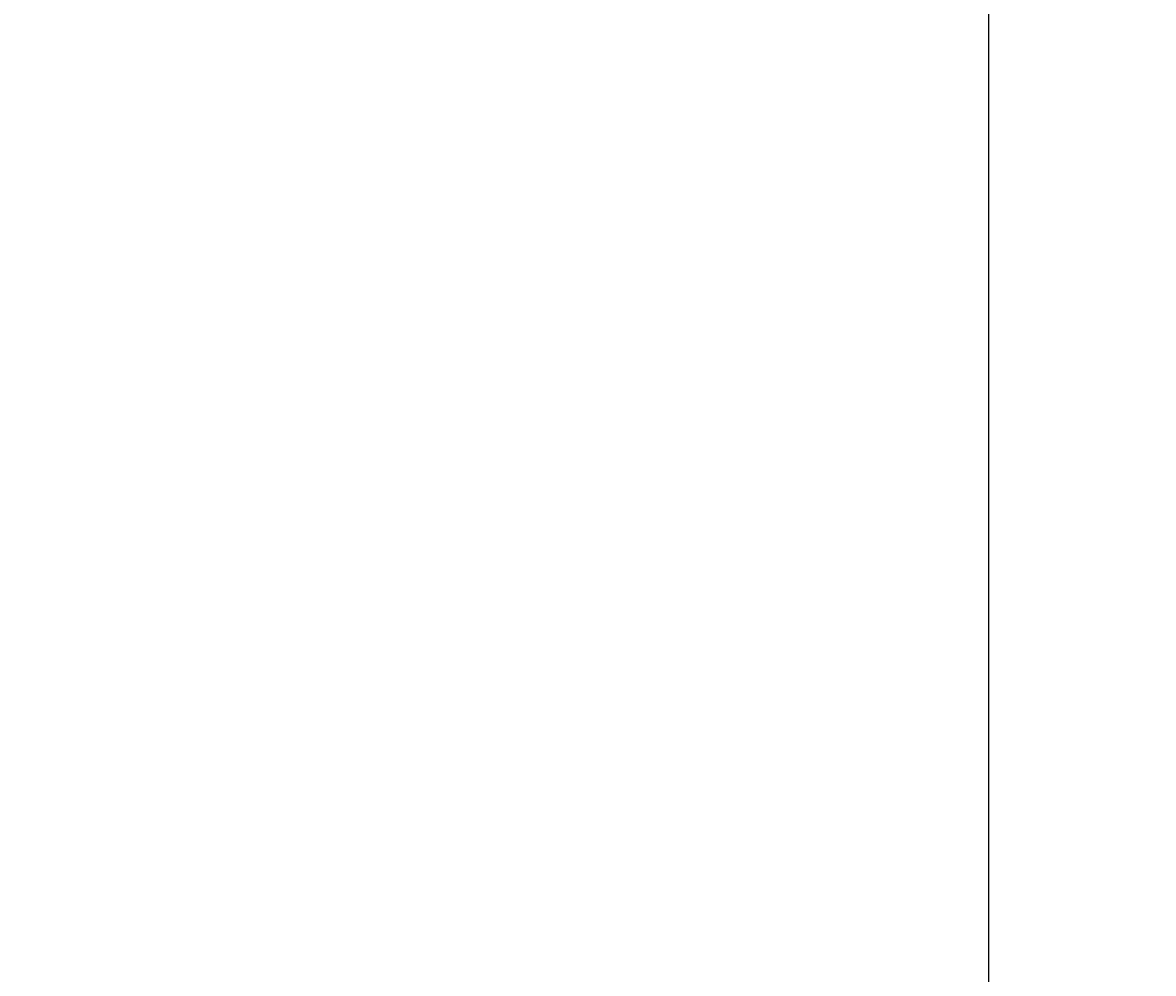
# Model space of a CAD drawing. Units: inches. Extents: x -61 to 1599, y -1316 to 257.
# Tile 48 of 204: x 149 to 185, y -478 to -447. Entities that reach past the tile are written whole.
import ezdxf

# ---------------------------------------------------------------- set-up
doc = ezdxf.new("R2010")
doc.units = ezdxf.units.IN
doc.header["$MEASUREMENT"] = 0
doc.layers.add('A-ANNO-DIMS', color=2, linetype='Continuous', lineweight=18)
doc.styles.get("Standard").update_dxf_attribs({"font": 'arial.ttf'})
doc.dimstyles.get("Standard").update_dxf_attribs({"dimtxt": 0.18, "dimasz": 0.18, "dimexe": 0.18, "dimexo": 0.0625, "dimgap": 0.09, "dimtad": 0, "dimtih": 1, "dimtoh": 1, "dimdec": 0, "dimzin": 0, "dimdsep": 46, "dimlunit": 3, "dimtxsty": 'Standard', "dimcen": 0.09, "dimadec": 0, "dimazin": 0, "dimtfac": 1, "dimtdec": 0, "dimtofl": 0, "dimtmove": 0, "dimatfit": 3, "dimfxl": 1, "dimtolj": 1, "dimtzin": 0, "dimarcsym": 0})

# ---------------------------------------------------------------- blocks, each defined once
blk = doc.blocks.new('*D687')
at = {"layer": 'A-ANNO-DIMS', "color": 0, "lineweight": -2, "transparency": 16777216}
for p, q in [((289.418, 181.677), (-61.077, 181.677)), ((-60.897, 181.497), (-60.897, -528.952)), ((-60.897, -1239.765), (-60.897, -529.316)), ((319.64, -1239.945), (-61.077, -1239.945))]:
    blk.add_line(p, q, dxfattribs=at)
at = {"layer": 'A-ANNO-DIMS', "color": 0, "transparency": 16777216}
for points in [[(-60.927, 181.497), (-60.867, 181.497), (-60.897, 181.677)], [(-60.927, -1239.765), (-60.867, -1239.765), (-60.897, -1239.945)]]:
    blk.add_solid(points, dxfattribs=at)
at = {"layer": 'DEFPOINTS', "color": 0, "transparency": 16777216}
for p in [(289.481, 181.677), (-60.897, -1239.945), (319.703, -1239.945)]:
    blk.add_point(p, dxfattribs=at)
at = {"layer": 'A-ANNO-DIMS', "color": 0, "transparency": 16777216, "insert": (-60.897, -529.134), "char_height": 0.18, "attachment_point": 5}
blk.add_mtext('\\A1;1421.6', dxfattribs=at)
blk = doc.blocks.new('*D700')
at = {"layer": 'A-ANNO-DIMS', "color": 0, "lineweight": -2, "transparency": 16777216}
for p, q in [((14.703, -616.882), (14.703, 257.457)), ((14.883, 257.277), (96.772, 257.277)), ((179.572, 257.277), (97.683, 257.277)), ((179.752, -616.882), (179.752, 257.457))]:
    blk.add_line(p, q, dxfattribs=at)
at = {"layer": 'A-ANNO-DIMS', "color": 0, "transparency": 16777216}
for points in [[(14.883, 257.307), (14.883, 257.247), (14.703, 257.277)], [(179.572, 257.307), (179.572, 257.247), (179.752, 257.277)]]:
    blk.add_solid(points, dxfattribs=at)
at = {"layer": 'DEFPOINTS', "color": 0, "transparency": 16777216}
for p in [(179.752, 257.277), (14.703, -616.945), (179.752, -616.945)]:
    blk.add_point(p, dxfattribs=at)
at = {"layer": 'A-ANNO-DIMS', "color": 0, "transparency": 16777216, "insert": (97.227, 257.277), "char_height": 0.18, "attachment_point": 5}
blk.add_mtext('\\A1;165.05', dxfattribs=at)

msp = doc.modelspace()

# ---------------------------------------------------------------- dimensions: what is measured, and where the dimension line sits
at = {"layer": 'A-ANNO-DIMS'}
dim = msp.add_linear_dim(base=(179.7521, 257.2771), p1=(14.7028, -616.9446), p2=(179.7521, -616.9446), dimstyle='Standard', override={"dimdec": 2, "dimlfac": 1, "dimrnd": 0, "dimzin": 0, "dimdsep": 46, "dimlunit": 2}, dxfattribs=at)
dim.commit()
dim.dimension.update_dxf_attribs({"geometry": '*D700', "text_midpoint": (97.2274, 257.2771)})
dim = msp.add_linear_dim(base=(-60.8972, -1239.9446), p1=(289.4807, 181.6771), p2=(319.7028, -1239.9446), angle=90, dimstyle='Standard', override={"dimdec": 1, "dimlfac": 1, "dimrnd": 0, "dimzin": 0, "dimdsep": 46, "dimlunit": 2}, dxfattribs=at)
dim.commit()
dim.dimension.update_dxf_attribs({"geometry": '*D687', "text_midpoint": (-60.8972, -529.1337)})

doc.saveas('drawing.dxf')
